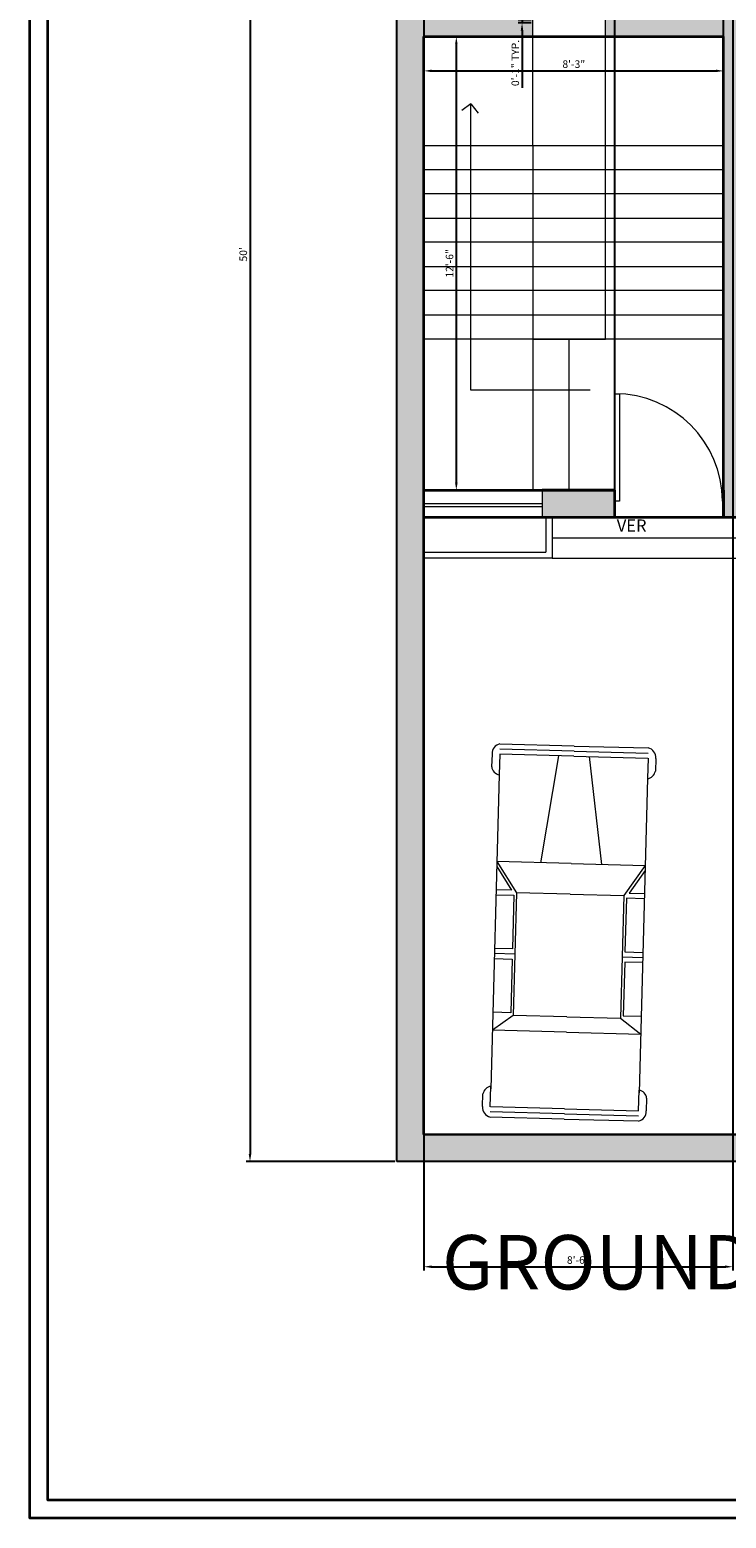
# Model space of a CAD drawing. Units: inches. Extents: x 2004 to 2661, y 1548 to 2351.
# Tile 1 of 5: x 2014 to 2244, y 1548 to 2040. Entities that reach past the tile are written whole.
import ezdxf

# ---------------------------------------------------------------- set-up
doc = ezdxf.new("R2010")
doc.units = ezdxf.units.IN
for name, color, linetype, lineweight in [('A-ANNO-DIMS', 2, 'Continuous', 18), ('A-ANNO-TEXT', 7, 'Continuous', 25), ('A-ANNO-TTLB', 7, 'Continuous', 35), ('A-AREA-IDEN', 7, 'Continuous', 18), ('A-DOOR', 3, 'Continuous', 18), ('A-EQPM-VEHI', 8, 'Continuous', 18), ('A-FLOR-STRS', 7, 'Continuous', 18), ('A-GLAZ', 4, 'Continuous', 18), ('A-WALL', 7, 'Continuous', 35), ('C-PROP', 7, 'Continuous', 25)]:
    doc.layers.add(name, color=color, linetype=linetype, lineweight=lineweight)
doc.layers.add('A-FLOR-PATT', color=18, linetype='Continuous', lineweight=13, true_color=0x000000)
doc.layers.add('A-WALL-PATT', color=18, linetype='Continuous', lineweight=13, true_color=0x000000)
doc.styles.get("Standard").update_dxf_attribs({"font": 'arial.ttf'})
doc.dimstyles.new('Copy of ISO-25', dxfattribs={"dimtxt": 2.5, "dimasz": 2.5, "dimexe": 1.25, "dimexo": 0.625, "dimtad": 1, "dimlunit": 4, "dimtxsty": 'Standard', "dimcen": 2.5, "dimadec": 0, "dimazin": 0, "dimtfac": 1, "dimtmove": 0, "dimatfit": 3, "dimfxl": 1, "dimarcsym": 0})

# ---------------------------------------------------------------- blocks, each defined once
blk = doc.blocks.new('*U5')
for p, q in [((0, 0), (0, -6)), ((40, 0), (40, -6))]:
    blk.add_line(p, q)
blk.add_lwpolyline([(0, 0), (0, 40), (1.75, 40), (1.75, 0)], close=True)
blk.add_arc((0, 0), 40, 0, 90)
blk = doc.blocks.new('*U12')
for p, q in [((138, 1075), (308, 1075)), ((4818, 1075), (4649, 1075)), ((3, -10), (3, 974)), ((70, -10), (70, 973)), ((138, 973), (410, 973)), ((138, -10), (138, 971)), ((410, 973), (4581, 973)), ((1563, -10), (1563, 973)), ((1563, 973), (1969, 702)), ((1630, 973), (1936, 769)), ((1936, 769), (1936, 973)), ((2003, 973), (2003, 736)), ((2716, 736), (2716, 973)), ((2783, 702), (2783, 973)), ((2851, 973), (2851, 736)), ((3563, 736), (3563, 973)), ((3597, 702), (3801, 973)), ((3801, -10), (3801, 973)), ((4818, 973), (4547, 973)), ((4818, -10), (4818, 971)), ((4886, -10), (4886, 973)), ((4954, -10), (4954, 974)), ((1969, 702), (3597, 702)), ((1969, -10), (1969, 702)), ((2003, 736), (2716, 736)), ((2851, 736), (3563, 736)), ((3597, -10), (3597, 702)), ((138, 193), (1563, 396)), ((3, -11), (3, -995)), ((70, -10), (70, -994)), ((138, -11), (138, -992)), ((1563, -10), (1563, -994)), ((1969, -10), (1969, -723)), ((3597, -10), (3597, -723)), ((3801, -10), (3801, -994)), ((4818, -11), (4818, -992)), ((4886, -10), (4886, -994)), ((4954, -11), (4954, -995)), ((138, -214), (1563, -417)), ((1563, -994), (1969, -723)), ((1969, -723), (3597, -723)), ((2003, -994), (2003, -757)), ((2003, -757), (2716, -757)), ((2716, -757), (2716, -994)), ((2783, -723), (2783, -994)), ((2851, -757), (3563, -757)), ((2851, -994), (2851, -757)), ((3563, -757), (3563, -994)), ((3597, -723), (3801, -994)), ((1630, -994), (1936, -790)), ((1936, -790), (1936, -994)), ((138, -994), (410, -994)), ((138, -1096), (308, -1096)), ((410, -994), (4581, -994)), ((4818, -994), (4547, -994)), ((4818, -1096), (4649, -1096))]:
    blk.add_line(p, q)
for centre, radius, start, end in [((128, 946), 129, 85.6455, 168.0943), ((291, 956), 120, 8.1301, 81.87), ((4665, 956), 120, 98.13, 171.8699), ((4828, 946), 129, 11.9057, 94.3545), ((128, -967), 129, 191.9057, 274.3545), ((291, -977), 120, 278.13, 351.8699), ((4665, -977), 120, 188.1301, 261.87), ((4828, -967), 129, 265.6455, 348.0943)]:
    blk.add_arc(centre, radius, start, end)
blk = doc.blocks.new('*D13')
at = {"layer": 'A-ANNO-DIMS', "color": 0, "lineweight": -2, "transparency": 16777216}
for p, q in [((2134.63, 2266.09), (2085.55, 2266.09)), ((2086.8, 2263.59), (2086.8, 1668.59)), ((2134.63, 1666.09), (2085.55, 1666.09))]:
    blk.add_line(p, q, dxfattribs=at)
at = {"layer": 'A-ANNO-DIMS', "color": 0, "transparency": 16777216}
for points in [[(2086.38, 2263.59), (2087.22, 2263.59), (2086.8, 2266.09)], [(2086.38, 1668.59), (2087.22, 1668.59), (2086.8, 1666.09)]]:
    blk.add_solid(points, dxfattribs=at)
at = {"layer": 'Defpoints', "color": 0, "transparency": 16777216}
for p in [(2135.26, 2266.09), (2086.8, 1666.09), (2135.26, 1666.09)]:
    blk.add_point(p, dxfattribs=at)
at = {"layer": 'A-ANNO-DIMS', "color": 0, "transparency": 16777216, "insert": (2084.9, 1966.09), "char_height": 2.5, "attachment_point": 5, "rotation": 90}
blk.add_mtext("50'", dxfattribs=at)
blk = doc.blocks.new('*D23')
at = {"layer": 'A-ANNO-DIMS', "color": 0, "lineweight": -2, "transparency": 16777216}
for p, q in [((2144.26, 2037.47), (2144.26, 2025.5)), ((2243.26, 2037.47), (2243.26, 2025.5)), ((2146.76, 2026.75), (2240.76, 2026.75))]:
    blk.add_line(p, q, dxfattribs=at)
at = {"layer": 'A-ANNO-DIMS', "color": 0, "transparency": 16777216}
for points in [[(2146.76, 2027.17), (2146.76, 2026.34), (2144.26, 2026.75)], [(2240.76, 2027.17), (2240.76, 2026.34), (2243.26, 2026.75)]]:
    blk.add_solid(points, dxfattribs=at)
at = {"layer": 'Defpoints', "color": 0, "transparency": 16777216}
for p in [(2144.26, 2038.09), (2243.26, 2038.09), (2243.26, 2026.75)]:
    blk.add_point(p, dxfattribs=at)
at = {"layer": 'A-ANNO-DIMS', "color": 0, "transparency": 16777216, "insert": (2193.76, 2028.66), "char_height": 2.5, "attachment_point": 5}
blk.add_mtext('8\'-3"', dxfattribs=at)
blk = doc.blocks.new('*D24')
at = {"layer": 'A-ANNO-DIMS', "color": 0, "lineweight": -2, "transparency": 16777216}
for p, q in [((2144.88, 2038.09), (2156.2, 2038.09)), ((2154.95, 2035.59), (2154.95, 1890.59)), ((2144.88, 1888.09), (2156.2, 1888.09))]:
    blk.add_line(p, q, dxfattribs=at)
at = {"layer": 'A-ANNO-DIMS', "color": 0, "transparency": 16777216}
for points in [[(2154.54, 2035.59), (2155.37, 2035.59), (2154.95, 2038.09)], [(2154.54, 1890.59), (2155.37, 1890.59), (2154.95, 1888.09)]]:
    blk.add_solid(points, dxfattribs=at)
at = {"layer": 'Defpoints', "color": 0, "transparency": 16777216}
for p in [(2144.26, 2038.09), (2144.26, 1888.09), (2154.95, 1888.09)]:
    blk.add_point(p, dxfattribs=at)
at = {"layer": 'A-ANNO-DIMS', "color": 0, "transparency": 16777216, "insert": (2153.05, 1963.09), "char_height": 2.5, "attachment_point": 5, "rotation": 90}
blk.add_mtext('12\'-6"', dxfattribs=at)
blk = doc.blocks.new('*D36')
at = {"layer": 'A-ANNO-DIMS', "color": 0, "lineweight": -2, "transparency": 16777216}
for p, q in [((2176.66, 2046.09), (2176.66, 2048.59)), ((2179.63, 2043.59), (2175.41, 2043.59)), ((2179.63, 2042.59), (2175.41, 2042.59)), ((2176.66, 2043.59), (2176.66, 2042.59)), ((2176.66, 2040.09), (2176.66, 2021.1))]:
    blk.add_line(p, q, dxfattribs=at)
at = {"layer": 'A-ANNO-DIMS', "color": 0, "transparency": 16777216}
for points in [[(2176.24, 2046.09), (2177.07, 2046.09), (2176.66, 2043.59)], [(2176.24, 2040.09), (2177.07, 2040.09), (2176.66, 2042.59)]]:
    blk.add_solid(points, dxfattribs=at)
at = {"layer": 'Defpoints', "color": 0, "transparency": 16777216}
for p in [(2176.66, 2042.59), (2180.26, 2043.59), (2180.26, 2042.59)]:
    blk.add_point(p, dxfattribs=at)
at = {"layer": 'A-ANNO-DIMS', "color": 0, "transparency": 16777216, "insert": (2174.76, 2029.35), "char_height": 2.5, "attachment_point": 5, "rotation": 90}
blk.add_mtext('0\'-1" TYP.', dxfattribs=at)
blk = doc.blocks.new('*D37')
at = {"layer": 'A-ANNO-DIMS', "color": 0, "lineweight": -2, "transparency": 16777216}
for p, q in [((2246.26, 2082.47), (2246.26, 1630.09)), ((2144.26, 2046.47), (2144.26, 1630.09)), ((2146.76, 1631.34), (2243.76, 1631.34))]:
    blk.add_line(p, q, dxfattribs=at)
at = {"layer": 'A-ANNO-DIMS', "color": 0, "transparency": 16777216}
for points in [[(2146.76, 1631.76), (2146.76, 1630.93), (2144.26, 1631.34)], [(2243.76, 1631.76), (2243.76, 1630.93), (2246.26, 1631.34)]]:
    blk.add_solid(points, dxfattribs=at)
at = {"layer": 'Defpoints', "color": 0, "transparency": 16777216}
for p in [(2246.26, 2083.09), (2144.26, 2047.09), (2246.26, 1631.34)]:
    blk.add_point(p, dxfattribs=at)
at = {"layer": 'A-ANNO-DIMS', "color": 0, "transparency": 16777216, "insert": (2195.26, 1633.24), "char_height": 2.5, "attachment_point": 5}
blk.add_mtext('8\'-6"', dxfattribs=at)
blk = doc.blocks.new('*D46')
at = {"layer": 'A-ANNO-DIMS', "color": 0, "lineweight": -2, "transparency": 16777216}
for p, q in [((2207.26, 1879.72), (2207.26, 2346.91)), ((2209.76, 2345.66), (2240.76, 2345.66)), ((2243.26, 1879.72), (2243.26, 2346.91))]:
    blk.add_line(p, q, dxfattribs=at)
at = {"layer": 'A-ANNO-DIMS', "color": 0, "transparency": 16777216}
for points in [[(2209.76, 2346.07), (2209.76, 2345.24), (2207.26, 2345.66)], [(2240.76, 2346.07), (2240.76, 2345.24), (2243.26, 2345.66)]]:
    blk.add_solid(points, dxfattribs=at)
at = {"layer": 'Defpoints', "color": 0, "transparency": 16777216}
for p in [(2243.26, 2345.66), (2207.26, 1879.09), (2243.26, 1879.09)]:
    blk.add_point(p, dxfattribs=at)
at = {"layer": 'A-ANNO-DIMS', "color": 0, "transparency": 16777216, "insert": (2225.26, 2347.56), "char_height": 2.5, "attachment_point": 5}
blk.add_mtext('3\'-0"', dxfattribs=at)

msp = doc.modelspace()

# ---------------------------------------------------------------- hatches: boundary and pattern name
at = {"layer": 'A-FLOR-PATT'}
h = msp.add_hatch(dxfattribs=at)
h.set_pattern_fill('ANSI32', color=256)
h.paths.add_polyline_path([(2522.257, 2257.093), (2466.833, 2257.093), (2315.257, 2257.093), (2418.757, 2233.093)])
h.paths.add_polyline_path([(2418.757, 2233.093), (2315.257, 2257.093), (2315.257, 2209.093)])
h.paths.add_polyline_path([(2418.757, 2233.093), (2315.257, 2209.093), (2522.257, 2209.093)])
h.paths.add_polyline_path([(2522.257, 2257.093), (2418.757, 2233.093), (2522.257, 2209.093)])
h.paths.add_polyline_path([(2522.257, 1753.093), (2318.257, 1753.093), (2318.257, 1675.093), (2522.257, 1675.093)])
h.paths.add_polyline_path([(2210.267, 2081.517), (2210.233, 2081.517), (2210.233, 2083.093), (2246.257, 2083.093), (2246.257, 2119.093), (2144.257, 2119.093), (2144.257, 2047.093), (2244.938, 2047.093, -0.390864)])
h.paths.add_polyline_path([(2171.613, 2077.721), (2161.069, 2080.96), (2161.193, 2075.729), (2163.808, 2075.791), (2163.932, 2070.56), (2162.189, 2070.519), (2162.106, 2074.006), (2161.234, 2073.986), (2161.338, 2069.627), (2147.389, 2069.296), (2146.521, 2105.911), (2160.469, 2106.241), (2160.738, 2094.908), (2171.117, 2098.643, -0.7025712), (2195.775, 2088.761, -0.7025621)], flags=16)
h.paths.add_polyline_path([(2171.53, 2081.208), (2171.2, 2095.156, -0.7345333), (2194.031, 2088.72, -0.7345297)], flags=0)
h.paths.add_polyline_path([(2158.245, 2071.298), (2150.835, 2071.122, -0.4142136), (2149.061, 2072.388), (2148.347, 2102.465, -0.4142136), (2149.614, 2104.239), (2157.024, 2104.415, -0.4142136), (2158.798, 2103.149), (2159.512, 2073.072, -0.4142136)], flags=0)
h.paths.add_polyline_path([(2522.257, 2200.093), (2517.397, 2200.093), (2517.397, 2185.232), (2505.384, 2185.232), (2509.08, 2174.143, -0.7025712), (2497.991, 2148.268, -0.7025621), (2486.902, 2174.142), (2490.599, 2185.232), (2485.054, 2185.232), (2485.054, 2182.459), (2479.509, 2182.459), (2479.509, 2184.307), (2483.206, 2184.307), (2483.206, 2185.232), (2478.585, 2185.232), (2478.585, 2200.093), (2459.257, 2200.093), (2459.257, 2106.686, -0.3761573), (2493.676, 2139.619), (2493.676, 2139.653), (2495.257, 2139.653), (2495.257, 2104.093), (2522.257, 2104.093)])
h.paths.add_polyline_path([(2349.854, 1719.146), (2381.921, 1719.146), (2381.921, 1725.273), (2349.854, 1725.273)], flags=24)
h.paths.add_polyline_path([(2349.84, 1725.558), (2388.851, 1725.558), (2388.851, 1731.767), (2349.84, 1731.767)], flags=24)
h.paths.add_polyline_path([(2152.908, 2086.679), (2181.867, 2086.679), (2181.867, 2092.806), (2152.908, 2092.806)], flags=8)
h.paths.add_polyline_path([(2152.895, 2093.091), (2174.525, 2093.091), (2174.525, 2099.3), (2152.895, 2099.3)], flags=8)
h.paths.add_polyline_path([(2515.001, 2150.174), (2515.001, 2154.033), (2509.85, 2154.033), (2509.85, 2150.174)], flags=24)
h.paths.add_polyline_path([(2469.272, 2171.563), (2498.231, 2171.563), (2498.231, 2177.69), (2469.272, 2177.69)], flags=24)
h.paths.add_polyline_path([(2469.258, 2177.975), (2490.888, 2177.975), (2490.888, 2184.184), (2469.258, 2184.184)], flags=24)
at = {"layer": 'A-WALL-PATT'}
h = msp.add_hatch(color=256, dxfattribs=at)
h.dxf.hatch_style = 1
h.paths.add_polyline_path([(2315.257, 2266.093), (2135.257, 2266.093), (2135.257, 1666.093), (2531.257, 1666.093), (2531.257, 1753.093), (2522.257, 1753.093), (2522.257, 1675.093), (2144.257, 1675.093), (2144.257, 2038.093), (2180.257, 2038.093), (2180.257, 2047.093), (2144.257, 2047.093), (2144.257, 2257.093), (2309.257, 2257.093), (2315.257, 2257.093)])
h.paths.add_polyline_path([(2522.257, 2266.093), (2315.257, 2266.093), (2315.257, 2257.093), (2522.257, 2257.093)], flags=17)
h.paths.add_polyline_path([(2368.773, 2209.093), (2315.257, 2209.093), (2309.257, 2209.093), (2309.257, 2119.093), (2309.257, 2083.093), (2315.257, 2083.093), (2315.257, 2119.093), (2315.257, 2200.093), (2368.773, 2200.093)], flags=17)
h.paths.add_polyline_path([(2459.257, 2209.093), (2428.773, 2209.093), (2428.773, 2200.093), (2453.257, 2200.093), (2459.257, 2200.093)], flags=17)
h.paths.add_polyline_path([(2522.257, 2209.093), (2483.257, 2209.093), (2483.257, 2200.093), (2522.257, 2200.093)], flags=17)
h.paths.add_polyline_path([(2522.257, 2044.093), (2459.257, 2044.093), (2459.257, 2056.073, -0.004139), (2458.66, 2056.069), (2453.257, 2056.069), (2453.257, 2044.093), (2315.257, 2044.093), (2315.257, 2046.941, -0.0039864), (2314.68, 2046.936), (2309.257, 2046.936), (2309.257, 2038.093), (2315.257, 2038.093), (2522.257, 2038.093)], flags=17)
h.paths.add_polyline_path([(2531.257, 2266.093), (2522.257, 2266.093), (2522.257, 2257.093), (2522.257, 2209.093), (2522.257, 2200.093), (2522.257, 2104.093), (2522.257, 1762.093), (2498.257, 1762.093), (2498.257, 1753.093), (2522.257, 1753.093), (2531.257, 1753.093)], flags=17)
h.paths.add_polyline_path([(2522.257, 2104.093), (2495.257, 2104.093), (2495.257, 2103.514), (2495.257, 2098.093), (2503.401, 2098.093), (2522.257, 2098.093)], flags=17)
h.paths.add_polyline_path([(2455.748, 2073.874), (2484.708, 2073.874), (2484.708, 2080.001), (2455.748, 2080.001)], flags=25)
h.paths.add_polyline_path([(2455.735, 2080.287), (2477.056, 2080.287), (2477.056, 2086.492), (2455.735, 2086.492)], flags=25)
h.paths.add_polyline_path([(2469.272, 2171.563), (2498.231, 2171.563), (2498.231, 2177.69), (2469.272, 2177.69)], flags=25)
h.paths.add_polyline_path([(2469.258, 2177.975), (2490.888, 2177.975), (2490.888, 2184.184), (2469.258, 2184.184)], flags=25)
h.paths.add_polyline_path([(2360.849, 2078.511), (2396.023, 2078.511), (2396.023, 2084.638), (2360.849, 2084.638)], flags=25)
h.paths.add_polyline_path([(2360.835, 2084.923), (2394.883, 2084.923), (2394.883, 2091.132), (2360.835, 2091.132)], flags=25)
h = msp.add_hatch(color=256, dxfattribs=at)
h.dxf.hatch_style = 1
h.paths.add_polyline_path([(2252.257, 2038.093), (2252.257, 2047.093), (2246.257, 2047.093), (2204.257, 2047.093), (2204.257, 2038.093), (2243.257, 2038.093), (2243.257, 1888.093), (2243.257, 1879.093), (2273.257, 1879.093), (2273.257, 1888.093), (2252.257, 1888.093)])
h.paths.add_polyline_path([(2273.257, 2125.093), (2144.257, 2125.093), (2144.257, 2119.093), (2246.257, 2119.093), (2273.257, 2119.093)])
h.paths.add_polyline_path([(2459.257, 2200.093), (2453.257, 2200.093), (2453.257, 2092.093), (2459.257, 2092.093)])
h.paths.add_polyline_path([(2522.257, 1888.093), (2426.257, 1888.093), (2426.257, 1882.093), (2522.257, 1882.093)])
h.paths.add_polyline_path([(2460.257, 1834.093), (2454.257, 1834.093), (2454.257, 1762.093), (2460.257, 1762.093)])
h.paths.add_polyline_path([(2460.257, 1882.093), (2454.257, 1882.093), (2454.257, 1870.093), (2460.257, 1870.093)])
h.paths.add_polyline_path([(2462.257, 1762.093), (2460.257, 1762.093), (2454.257, 1762.093), (2390.257, 1762.093), (2390.257, 1753.093), (2462.257, 1753.093)])
h.paths.add_polyline_path([(2342.257, 1762.093), (2318.257, 1762.093), (2318.257, 1882.093), (2318.257, 1888.093), (2309.257, 1888.093), (2309.257, 1879.093), (2309.257, 1753.093), (2318.257, 1753.093), (2342.257, 1753.093)])
h.paths.add_polyline_path([(2354.257, 1888.093), (2318.257, 1888.093), (2318.257, 1882.093), (2354.257, 1882.093)])
h.paths.add_polyline_path([(2318.257, 1753.093), (2309.257, 1753.093), (2309.257, 1675.093), (2318.257, 1675.093)])
h.paths.add_polyline_path([(2207.257, 1884.43), (2207.257, 1888.093), (2183.257, 1888.093), (2183.257, 1879.093), (2207.257, 1879.093)])
h.paths.add_polyline_path([(2252.257, 2119.093), (2246.257, 2119.093), (2246.257, 2083.093), (2251.66, 2083.093), (2252.257, 2083.093)])
h.paths.add_polyline_path([(2315.257, 2257.093), (2309.257, 2257.093), (2309.257, 2209.093), (2315.257, 2209.093)])

# ---------------------------------------------------------------- linework, layer by layer
at = {"layer": 'A-ANNO-TTLB'}
for points in [[(2014.058, 2344.754), (2661.447, 2344.754), (2661.447, 1548.19), (2014.058, 1548.19)], [(2020.058, 2338.754), (2655.447, 2338.754), (2655.447, 1554.19), (2020.058, 1554.19)]]:
    msp.add_lwpolyline(points, close=True, dxfattribs=at)
at = {"layer": 'A-FLOR-STRS'}
for p, q in [((2144.257, 2038.093), (2144.257, 2002.093)), ((2180.257, 2002.093), (2180.257, 2038.093)), ((2204.257, 2002.093), (2204.257, 2038.093)), ((2159.779, 2015.857), (2156.812, 2013.621)), ((2159.779, 1921.169), (2159.779, 2015.857)), ((2159.779, 2015.857), (2162.123, 2012.747)), ((2144.257, 2002.093), (2243.257, 2002.093)), ((2144.257, 2002.093), (2144.257, 1994.093)), ((2144.257, 2002.093), (2180.257, 2002.093)), ((2180.257, 2002.093), (2180.257, 1938.093)), ((2204.257, 1938.093), (2204.257, 2002.093)), ((2144.257, 1994.093), (2243.257, 1994.093)), ((2243.257, 1994.093), (2243.257, 1986.093)), ((2243.257, 1986.093), (2144.257, 1986.093)), ((2144.257, 1986.093), (2144.257, 1978.093)), ((2144.257, 1978.093), (2243.257, 1978.093)), ((2243.257, 1978.093), (2243.257, 1970.093)), ((2243.257, 1970.093), (2144.257, 1970.093)), ((2144.257, 1970.093), (2144.257, 1962.093)), ((2144.257, 1962.093), (2243.257, 1962.093)), ((2243.257, 1962.093), (2243.257, 1954.093)), ((2243.257, 1954.093), (2144.257, 1954.093)), ((2144.257, 1954.093), (2144.257, 1946.093)), ((2144.257, 1946.093), (2243.257, 1946.093)), ((2243.257, 1946.093), (2243.257, 1938.093)), ((2243.257, 1938.093), (2144.257, 1938.093)), ((2180.257, 1938.093), (2204.257, 1938.093)), ((2180.257, 1938.093), (2180.257, 1888.093)), ((2192.257, 1888.093), (2192.257, 1938.093)), ((2199.126, 1921.169), (2159.779, 1921.169)), ((2180.257, 1888.093), (2192.257, 1888.093)), ((2183.257, 1879.093), (2186.568, 1879.093)), ((2186.568, 1879.093), (2184.568, 1879.093)), ((2184.568, 1879.093), (2184.568, 1867.618)), ((2186.568, 1879.093), (2186.568, 1865.618)), ((2186.568, 1872.355), (2257.874, 1872.355)), ((2144.257, 1865.618), (2144.257, 1867.618)), ((2144.257, 1867.618), (2184.568, 1867.618)), ((2186.568, 1865.618), (2144.257, 1865.618)), ((2186.568, 1865.618), (2257.874, 1865.618))]:
    msp.add_line(p, q, dxfattribs=at)
at = {"layer": 'A-GLAZ'}
for p, q in [((2180.257, 2038.093), (2180.257, 2047.093)), ((2204.257, 2038.093), (2204.257, 2047.093)), ((2144.257, 1879.093), (2144.257, 1888.093)), ((2183.257, 1888.093), (2183.257, 1879.093)), ((2183.257, 1883.593), (2144.257, 1883.593)), ((2144.257, 1883.593), (2144.257, 1883.593)), ((2183.257, 1882.593), (2144.257, 1882.593))]:
    msp.add_line(p, q, dxfattribs=at)
at = {"layer": 'A-WALL'}
for p, q in [((2144.257, 1675.093), (2144.257, 2038.093)), ((2144.257, 2038.093), (2243.257, 2038.093)), ((2243.257, 1888.093), (2243.257, 2038.093)), ((2144.257, 1888.093), (2207.257, 1888.093)), ((2207.257, 1888.093), (2183.257, 1888.093)), ((2207.257, 1888.093), (2207.257, 1879.093)), ((2243.257, 1888.093), (2243.257, 1879.093)), ((2309.257, 1879.093), (2144.257, 1879.093))]:
    msp.add_line(p, q, dxfattribs=at)
at = {"layer": 'C-PROP'}
for p, q in [((2135.257, 1666.093), (2135.257, 2266.093)), ((2522.257, 1675.093), (2144.257, 1675.093)), ((2144.257, 1675.093), (2309.257, 1675.093)), ((2531.257, 1666.093), (2135.257, 1666.093))]:
    msp.add_line(p, q, dxfattribs=at)

# ---------------------------------------------------------------- block references
at = {"layer": 'A-DOOR', "xscale": 0.8895088189668753, "yscale": 0.8895088189668753, "zscale": 0.8895088189668753}
msp.add_blockref('*U5', (2207.257, 1884.43), dxfattribs=at)
at = {"layer": 'A-EQPM-VEHI', "xscale": 0.0249183822300443, "yscale": 0.0249183822300443, "zscale": 0.0249183822300443, "rotation": 268.4785815451888}
msp.add_blockref('*U12', (2194.132, 1803.583), dxfattribs=at)

# ---------------------------------------------------------------- texts
at = {"layer": 'A-ANNO-TEXT'}
msp.add_text('GROUND FLOOR PLAN', height=18, dxfattribs=at).set_placement((2150.24, 1623.82))
at = {"layer": 'A-AREA-IDEN'}
msp.add_text('VER', height=4, dxfattribs=at).set_placement((2207.956, 1874.424))

# ---------------------------------------------------------------- dimensions: what is measured, and where the dimension line sits
at = {"layer": 'A-ANNO-DIMS'}
for base, p1, p2, override, picture, middle in [((2243.257, 2345.658), (2207.257, 1879.093), (2243.257, 1879.093), {"dimdec": 1, "dimlfac": 1, "dimrnd": 0, "dimzin": 1, "dimdsep": 46, "dimlunit": 4, "dimfrac": 2}, '*D46', (2225.257, 2347.56)), ((2246.257, 1631.343), (2144.257, 2047.093), (2246.257, 2083.093), {"dimdec": 1, "dimlfac": 1, "dimrnd": 0, "dimzin": 1, "dimdsep": 46, "dimlunit": 4, "dimfrac": 2}, '*D37', (2195.257, 1633.244)), ((2243.257, 2026.754), (2144.257, 2038.093), (2243.257, 2038.093), {"dimclrd": 0, "dimclre": 0, "dimclrt": 0}, '*D23', (2193.757, 2028.656))]:
    dim = msp.add_linear_dim(base=base, p1=p1, p2=p2, dimstyle='Copy of ISO-25', override=override, dxfattribs=at)
    dim.commit()
    dim.dimension.update_dxf_attribs({"geometry": picture, "text_midpoint": middle})
for base, p1, p2, picture, middle in [((2086.8, 1666.093), (2135.257, 2266.093), (2135.257, 1666.093), '*D13', (2084.899, 1966.093)), ((2154.954, 1888.093), (2144.257, 2038.093), (2144.257, 1888.093), '*D24', (2153.053, 1963.093))]:
    dim = msp.add_linear_dim(base=base, p1=p1, p2=p2, angle=90, dimstyle='Copy of ISO-25', override={"dimclrd": 0, "dimclre": 0, "dimclrt": 0}, dxfattribs=at)
    dim.commit()
    dim.dimension.update_dxf_attribs({"geometry": picture, "text_midpoint": middle})
dim = msp.add_linear_dim(base=(2176.657, 2042.593), p1=(2180.257, 2043.593), p2=(2180.257, 2042.593), angle=270, text='<> TYP.', dimstyle='Copy of ISO-25', override={"dimdec": 1, "dimlfac": 1, "dimrnd": 0, "dimzin": 1, "dimdsep": 46, "dimlunit": 4, "dimfrac": 2}, dxfattribs=at)
dim.commit()
dim.dimension.update_dxf_attribs({"geometry": '*D36', "text_midpoint": (2174.755, 2029.348)})

doc.saveas('drawing.dxf')
